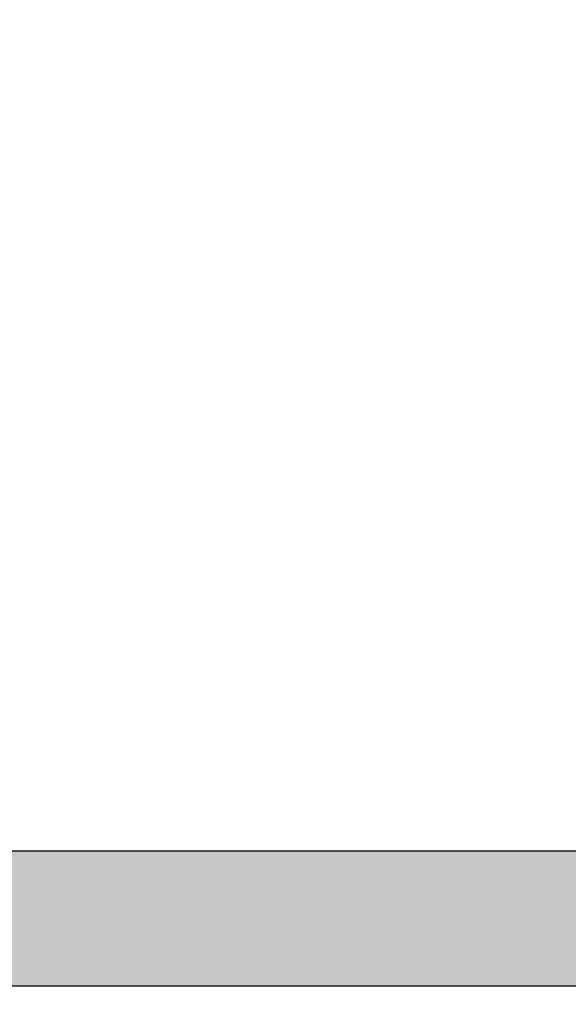
# Model space of a CAD drawing. Units: millimetres. Extents: x 7894 to 8038, y 6851 to 6951.
# Tile 20 of 49: x 7954.632 to 7956.664, y 6906.405 to 6910.053. Entities that reach past the tile are written whole.
import ezdxf

# ---------------------------------------------------------------- set-up
doc = ezdxf.new("R2010")
doc.units = ezdxf.units.MM
doc.layers.add('A-ANNO-DIMS', color=2, linetype='Continuous', lineweight=18)
doc.layers.add('A-FURN-SHLF', color=7, linetype='Continuous', lineweight=30)
doc.layers.add('A-FURN-PATT', color=32, linetype='Continuous', lineweight=9, true_color=0xcd6928)
doc.styles.get("Standard").update_dxf_attribs({"font": 'arial.ttf'})
doc.dimstyles.new('ISO-25', dxfattribs={"dimtxt": 1, "dimasz": 1, "dimexe": 1.25, "dimexo": 0.625, "dimtad": 1, "dimdec": 0, "dimlunit": 4, "dimtxsty": 'Standard', "dimcen": 2.5, "dimclrt": 1, "dimadec": 0, "dimazin": 0, "dimtfac": 1, "dimtdec": 0, "dimtmove": 0, "dimatfit": 3, "dimfxl": 1, "dimarcsym": 0})

# ---------------------------------------------------------------- blocks, each defined once
blk = doc.blocks.new('*D23')
at = {"layer": 'A-ANNO-DIMS', "color": 0, "lineweight": -2, "transparency": 16777216}
for p, q in [((7940.0888, 6907.098), (7940.0888, 6947.7928)), ((7971.9356, 6928.989), (7971.9356, 6947.7928)), ((7941.0888, 6946.5428), (7970.9356, 6946.5428))]:
    blk.add_line(p, q, dxfattribs=at)
at = {"layer": 'A-ANNO-DIMS', "color": 0, "transparency": 16777216}
for points in [[(7941.0888, 6946.7095), (7941.0888, 6946.3762), (7940.0888, 6946.5428)], [(7970.9356, 6946.7095), (7970.9356, 6946.3762), (7971.9356, 6946.5428)]]:
    blk.add_solid(points, dxfattribs=at)
at = {"layer": 'Defpoints', "color": 0, "transparency": 16777216}
for p in [(7971.9356, 6946.5428), (7971.9356, 6928.364), (7940.0888, 6906.473)]:
    blk.add_point(p, dxfattribs=at)
at = {"layer": 'A-ANNO-DIMS', "color": 1, "transparency": 16777216, "insert": (7956.0122, 6947.6784), "char_height": 1, "attachment_point": 5}
blk.add_mtext('2\'-8"', dxfattribs=at)
blk = doc.blocks.new('*D25')
at = {"layer": 'A-ANNO-DIMS', "color": 0, "lineweight": -2, "transparency": 16777216}
for p, q in [((7940.0888, 6905.848), (7940.0888, 6903.2865)), ((7964.3408, 6905.8484), (7964.3408, 6903.2865)), ((7941.0888, 6904.5365), (7963.3408, 6904.5365))]:
    blk.add_line(p, q, dxfattribs=at)
at = {"layer": 'A-ANNO-DIMS', "color": 0, "transparency": 16777216}
for points in [[(7941.0888, 6904.7032), (7941.0888, 6904.3699), (7940.0888, 6904.5365)], [(7963.3408, 6904.7032), (7963.3408, 6904.3699), (7964.3408, 6904.5365)]]:
    blk.add_solid(points, dxfattribs=at)
at = {"layer": 'Defpoints', "color": 0, "transparency": 16777216}
for p in [(7940.0888, 6906.473), (7964.3408, 6906.4734), (7964.3408, 6904.5365)]:
    blk.add_point(p, dxfattribs=at)
at = {"layer": 'A-ANNO-DIMS', "color": 1, "transparency": 16777216, "insert": (7952.2148, 6905.6786), "char_height": 1, "attachment_point": 5}
blk.add_mtext('2\'-0 1/2"', dxfattribs=at)
blk = doc.blocks.new('*D26')
at = {"layer": 'A-ANNO-DIMS', "color": 0, "lineweight": -2, "transparency": 16777216}
for p, q in [((7950.9654, 6918.7198), (7975.2272, 6918.7198)), ((7973.9772, 6917.7198), (7973.9772, 6907.4734)), ((7964.9658, 6906.4734), (7975.2272, 6906.4734))]:
    blk.add_line(p, q, dxfattribs=at)
at = {"layer": 'A-ANNO-DIMS', "color": 0, "transparency": 16777216}
for points in [[(7973.8105, 6917.7198), (7974.1439, 6917.7198), (7973.9772, 6918.7198)], [(7973.8105, 6907.4734), (7974.1439, 6907.4734), (7973.9772, 6906.4734)]]:
    blk.add_solid(points, dxfattribs=at)
at = {"layer": 'Defpoints', "color": 0, "transparency": 16777216}
for p in [(7950.3404, 6918.7198), (7964.3408, 6906.4734), (7973.9772, 6906.4734)]:
    blk.add_point(p, dxfattribs=at)
at = {"layer": 'A-ANNO-DIMS', "color": 1, "transparency": 16777216, "insert": (7972.8416, 6912.5966), "char_height": 1, "attachment_point": 5, "rotation": 90}
blk.add_mtext('1\'-0"', dxfattribs=at)

msp = doc.modelspace()

# ---------------------------------------------------------------- hatches: boundary and pattern name
at = {"layer": 'A-FURN-PATT'}
h = msp.add_hatch(color=256, dxfattribs=at)
h.dxf.hatch_style = 1
h.paths.add_polyline_path([(7942.8406, 6913.3629), (7942.8593, 6913.356), (7942.8677, 6913.356), (7942.8677, 6914.2132), (7942.876, 6914.2376), (7942.8813, 6914.2376), (7942.9022, 6914.2457), (7943.3657, 6914.2457), (7943.3844, 6914.2376), (7943.3861, 6914.2376), (7943.3858, 6914.2132), (7943.3852, 6913.2312), (7943.3944, 6906.9948), (7943.387, 6906.9732), (7943.4027, 6906.9732), (7943.403, 6906.9948), (7943.4029, 6908.4372), (7943.3944, 6914.2132), (7943.4169, 6914.2376), (7943.4198, 6914.2457), (7943.4555, 6914.2457), (7943.4603, 6914.238), (7943.8607, 6914.2452), (7943.8615, 6914.2457), (7943.8623, 6914.2452), (7943.8866, 6914.2457), (7943.8944, 6914.2402), (7943.9104, 6914.2376), (7943.9211, 6914.2132), (7943.9294, 6914.2376), (7943.9318, 6914.2376), (7943.9453, 6914.2398), (7943.9488, 6914.2457), (7943.9797, 6914.2452), (7943.9807, 6914.2457), (7943.9815, 6914.2451), (7944.3738, 6914.2376), (7944.3882, 6914.2457), (7944.4201, 6914.2457), (7944.4341, 6914.2376), (7944.4395, 6914.2376), (7944.4478, 6914.2132), (7944.4478, 6914.1031), (7944.4622, 6914.099), (7944.7359, 6914.1607), (7944.8923, 6914.2014), (7944.9541, 6914.2098), (7944.955, 6914.21), (7946.556, 6907.1325), (7946.5534, 6907.1122), (7946.5529, 6907.1152), (7946.499, 6907.103), (7946.3343, 6907.0604), (7946.0282, 6906.9914), (7945.6731, 6908.5712), (7944.4484, 6914.0015), (7944.4478, 6906.9948), (7944.4404, 6906.9732), (7947.0373, 6906.9734), (7964.3408, 6906.9734), (7964.3408, 6906.4734), (7947.0373, 6906.4734), (7940.0888, 6906.473), (7940.0888, 6906.973), (7941.9951, 6906.9731), (7941.9899, 6906.9898), (7941.9899, 6913.3353), (7941.9968, 6913.3574), (7942.003, 6913.3571), (7942.0169, 6913.3629), (7942.0366, 6913.3629), (7942.0378, 6913.3629), (7942.0479, 6913.356), (7942.8142, 6913.356), (7942.8157, 6913.356), (7942.8346, 6913.356)])
h.paths.add_polyline_path([(7942.8598, 6913.0201), (7942.861, 6913.3353), (7942.8677, 6906.9948), (7942.876, 6906.9759), (7942.876, 6906.9903), (7942.8813, 6914.2376), (7942.876, 6914.2321), (7942.876, 6914.2177), (7942.8809, 6906.9647), (7942.8784, 6906.9704), (7942.876, 6906.9704), (7942.8574, 6906.9704), (7942.8613, 6911.8549)], flags=16)
h.paths.add_polyline_path([(7942.8613, 6911.8549), (7942.8677, 6906.9948), (7942.8686, 6906.9921), (7942.8677, 6906.9898), (7942.8616, 6906.9704), (7942.8598, 6906.9704), (7942.8574, 6906.9704), (7942.0002, 6906.9704), (7941.9978, 6906.9704), (7941.996, 6906.9704), (7941.9899, 6906.9898), (7941.9978, 6906.9704), (7942.0002, 6906.9704), (7942.8598, 6906.9704), (7942.8616, 6906.9748)], flags=16)
h.paths.add_polyline_path([(7942.023, 6913.356), (7942.0169, 6913.3629), (7942.0366, 6913.3629), (7942.0378, 6913.3629), (7942.0367, 6913.3614), (7942.0369, 6913.356)], flags=16)
h.paths.add_polyline_path([(7942.0366, 6913.3629), (7942.0169, 6913.3629), (7942.0196, 6913.3598)], flags=0)
h.paths.add_polyline_path([(7942.0353, 6913.356), (7942.0369, 6913.356), (7942.0367, 6913.3614)], flags=0)
h.paths.add_polyline_path([(7943.9293, 6906.9759), (7943.9211, 6906.9948), (7943.9294, 6906.9704)], flags=0)
h.paths.add_polyline_path([(7943.9125, 6914.2132), (7943.8982, 6914.2376), (7943.8944, 6914.2402), (7943.8832, 6914.2421), (7943.8781, 6914.2367), (7943.8765, 6914.2376), (7943.8789, 6914.2376), (7943.8866, 6914.2457), (7943.8623, 6914.2452), (7943.8607, 6914.2452), (7943.8615, 6914.2457), (7943.8623, 6914.2452), (7943.8866, 6914.2457), (7943.8944, 6914.2402), (7943.8982, 6914.2376), (7943.9097, 6914.218), (7943.9125, 6914.2168), (7943.9079, 6906.9704), (7943.9104, 6906.9704), (7943.9211, 6914.2132), (7943.9294, 6914.2376), (7943.9318, 6914.2376), (7943.9453, 6914.2398), (7943.9488, 6914.2457), (7943.9797, 6914.2452), (7943.9807, 6914.2457), (7943.9815, 6914.2451), (7944.3738, 6914.2376), (7944.3882, 6914.2457), (7944.4201, 6914.2457), (7944.4341, 6914.2376), (7944.4395, 6914.2376), (7944.4395, 6914.2177), (7944.4341, 6914.0941), (7944.4478, 6914.1004), (7944.4513, 6914.1021), (7944.4622, 6914.099), (7944.4343, 6914.0927), (7944.429, 6914.0915), (7944.4341, 6914.069), (7944.4484, 6914.0015), (7944.4341, 6914.0649), (7944.4346, 6906.9704), (7944.4371, 6906.9704), (7944.4395, 6906.9759), (7944.4395, 6906.9704), (7943.931, 6906.9704), (7943.9128, 6906.9704), (7943.9079, 6906.9704)], flags=16)
h.paths.add_polyline_path([(7943.9211, 6914.2132), (7943.9294, 6914.2376), (7943.9318, 6914.2376), (7943.9453, 6914.2398), (7943.9488, 6914.2457), (7943.9797, 6914.2452), (7943.9807, 6914.2457), (7943.9815, 6914.2451), (7944.3738, 6914.2376), (7944.3882, 6914.2457), (7944.4201, 6914.2457), (7944.4321, 6914.2387), (7944.4249, 6914.2376), (7944.4041, 6914.2376), (7944.4032, 6914.2136), (7944.4032, 6914.2376), (7944.4025, 6914.2379), (7944.3897, 6914.2382), (7944.3753, 6914.2384), (7944.3738, 6914.2376), (7943.9815, 6914.2451), (7943.9488, 6914.2457), (7943.9453, 6914.2398), (7943.9294, 6914.2132), (7943.931, 6906.9721), (7943.931, 6906.9704), (7943.9294, 6906.9704), (7943.9293, 6906.9759), (7943.9294, 6914.2132), (7943.9439, 6914.2376), (7943.9318, 6914.2376)], flags=0)
h.paths.add_polyline_path([(7942.8813, 6914.2376), (7942.8778, 6914.2362), (7942.8796, 6914.2404), (7942.885, 6914.239)], flags=17)
h.paths.add_polyline_path([(7944.4116, 6914.242), (7944.4104, 6914.2408), (7944.4125, 6914.2418)], flags=0)
h.paths.add_polyline_path([(7944.3879, 6914.2382), (7944.3882, 6914.2457), (7944.4094, 6914.241), (7944.4103, 6914.2408), (7944.4036, 6914.2373), (7944.39, 6914.2447), (7944.3897, 6914.2382)], flags=0)
h.paths.add_polyline_path([(7963.1359, 6906.9526), (7963.1396, 6906.9526), (7963.1431, 6906.9582)], flags=16)
h.paths.add_polyline_path([(7954.3975, 6907.3902), (7954.397, 6907.3948), (7954.3984, 6907.4007), (7954.3975, 6907.567), (7954.3984, 6907.5978), (7954.3986, 6907.7694), (7954.3978, 6907.7989), (7954.399, 6907.8759), (7954.3992, 6907.9037), (7954.3944, 6907.9081), (7954.4019, 6907.9055), (7954.3996, 6907.93), (7954.3988, 6907.9307), (7954.3841, 6907.9429), (7946.6754, 6907.9429), (7946.6535, 6907.9232), (7946.6531, 6907.9127), (7946.6527, 6907.7694), (7946.6525, 6907.4007), (7946.653, 6907.1185), (7946.6574, 6907.1224), (7946.656, 6907.1145), (7946.6571, 6907.1135), (7946.6675, 6907.1209), (7946.7515, 6907.1209), (7946.9105, 6907.1209), (7954.3003, 6907.1209), (7954.3895, 6907.1209), (7954.3915, 6907.1191), (7954.3991, 6907.1209), (7954.399, 6907.1383), (7954.3978, 6907.2163), (7954.3986, 6907.2413)], flags=17)
h.paths.add_polyline_path([(7954.3003, 6907.1209), (7954.3003, 6907.1136), (7946.9105, 6907.1129), (7946.7516, 6907.1136), (7946.7515, 6907.1209), (7946.6675, 6907.1209), (7946.6531, 6907.1106), (7946.653, 6907.1185), (7946.6574, 6907.1224), (7946.656, 6907.1145), (7946.6571, 6907.1135), (7946.6675, 6907.1209), (7946.7515, 6907.1209), (7946.9105, 6907.1209)], flags=17)
h.paths.add_polyline_path([(7954.3981, 6907.9048), (7954.3944, 6907.9081), (7954.3997, 6907.9062), (7954.4007, 6907.9186), (7954.4019, 6907.9055), (7954.405, 6907.9072), (7954.4044, 6907.9046), (7954.4027, 6907.8974), (7954.4024, 6907.9009), (7954.3996, 6907.9034), (7954.3996, 6907.9025), (7954.3994, 6907.9023), (7954.3995, 6907.9035)], flags=17)

# ---------------------------------------------------------------- linework, layer by layer
at = {"layer": 'A-FURN-SHLF'}
for p, q in [((7947.0373, 6906.9734), (7964.3408, 6906.9734)), ((7947.0373, 6906.4734), (7964.3408, 6906.4734))]:
    msp.add_line(p, q, dxfattribs=at)

# ---------------------------------------------------------------- dimensions: what is measured, and where the dimension line sits
at = {"layer": 'A-ANNO-DIMS'}
for base, p2, picture, middle in [((7971.9356, 6946.5428), (7971.9356, 6928.364), '*D23', (7956.0122, 6947.6784)), ((7964.3408, 6904.5365), (7964.3408, 6906.4734), '*D25', (7952.2148, 6905.6786))]:
    dim = msp.add_linear_dim(base=base, p1=(7940.0888, 6906.473), p2=p2, dimstyle='ISO-25', override={"dimdec": 1, "dimlfac": 1, "dimrnd": 0, "dimzin": 1, "dimdsep": 46, "dimlunit": 4, "dimfrac": 2}, dxfattribs=at)
    dim.commit()
    dim.dimension.update_dxf_attribs({"geometry": picture, "text_midpoint": middle})
dim = msp.add_linear_dim(base=(7973.9772, 6906.4734), p1=(7950.3404, 6918.7198), p2=(7964.3408, 6906.4734), angle=90, dimstyle='ISO-25', override={"dimdec": 1, "dimlfac": 1, "dimrnd": 0, "dimzin": 1, "dimdsep": 46, "dimlunit": 4, "dimfrac": 2}, dxfattribs=at)
dim.commit()
dim.dimension.update_dxf_attribs({"geometry": '*D26', "text_midpoint": (7972.8416, 6912.5966)})

doc.saveas('drawing.dxf')
